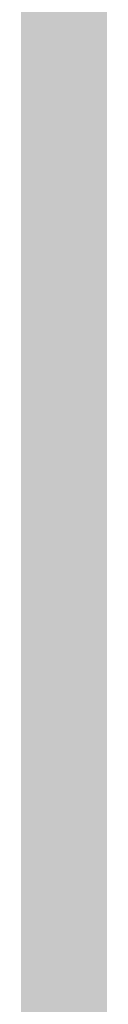
# Model space of a CAD drawing. Units: inches. Extents: x 2083 to 3317, y 1141 to 2115.
# Tile 173 of 256: x 3126.95825 to 3126.9594, y 1263.27402 to 1263.29018. Entities that reach past the tile are written whole.
import ezdxf

# ---------------------------------------------------------------- set-up
doc = ezdxf.new("R2010")
doc.units = ezdxf.units.IN
doc.layers.add('A-ANNO-DIMS', color=2, linetype='Continuous', lineweight=18)
doc.layers.add('A-WALL-PATT', color=251, linetype='Continuous', lineweight=13, true_color=0x636466)
doc.styles.get("Standard").update_dxf_attribs({"font": 'arial.ttf'})
doc.dimstyles.new('ISO-25', dxfattribs={"dimtxt": 12, "dimasz": 12, "dimexe": 1.25, "dimexo": 0.625, "dimtad": 1, "dimlunit": 3, "dimtxsty": 'Standard', "dimcen": 2.5, "dimadec": 0, "dimazin": 0, "dimtfac": 1, "dimtmove": 0, "dimatfit": 3, "dimfxl": 1, "dimarcsym": 0})

# ---------------------------------------------------------------- blocks, each defined once
blk = doc.blocks.new('*D26')
at = {"layer": 'A-ANNO-DIMS', "color": 0, "lineweight": -2, "transparency": 16777216}
for p, q in [((3088.985844, 1274.915092), (3088.985844, 1270.951963)), ((3111.240037, 1274.915092), (3111.240037, 1270.951963)), ((3076.985844, 1272.201963), (2840.262447, 1272.201963)), ((3111.240037, 1272.201963), (3088.985844, 1272.201963)), ((3123.240037, 1272.201963), (3135.240037, 1272.201963))]:
    blk.add_line(p, q, dxfattribs=at)
at = {"layer": 'A-ANNO-DIMS', "color": 0, "transparency": 16777216}
for points in [[(3076.985844, 1274.201963), (3076.985844, 1270.201963), (3088.985844, 1272.201963)], [(3123.240037, 1274.201963), (3123.240037, 1270.201963), (3111.240037, 1272.201963)]]:
    blk.add_solid(points, dxfattribs=at)
at = {"layer": 'Defpoints', "color": 0, "transparency": 16777216}
for p in [(3088.985844, 1275.540092), (3111.240037, 1275.540092), (3088.985844, 1272.201963)]:
    blk.add_point(p, dxfattribs=at)
at = {"layer": 'A-ANNO-DIMS', "color": 0, "transparency": 16777216, "insert": (2952.624146, 1279.031602), "char_height": 12, "attachment_point": 5}
blk.add_mtext('NIGHTSTAND 1\'-10 1/2" TYP.', dxfattribs=at)
blk = doc.blocks.new('*D27')
at = {"layer": 'A-ANNO-DIMS', "color": 0, "lineweight": -2, "transparency": 16777216}
for p, q in [((3114.578165, 1309.794285), (3114.578165, 1321.794285)), ((3111.865037, 1297.794285), (3115.828165, 1297.794285)), ((3114.578165, 1297.794285), (3114.578165, 1275.540092)), ((3111.865037, 1275.540092), (3115.828165, 1275.540092)), ((3114.578165, 1263.540092), (3114.578165, 1140.988591))]:
    blk.add_line(p, q, dxfattribs=at)
at = {"layer": 'A-ANNO-DIMS', "color": 0, "transparency": 16777216}
for points in [[(3112.578165, 1309.794285), (3116.578165, 1309.794285), (3114.578165, 1297.794285)], [(3112.578165, 1263.540092), (3116.578165, 1263.540092), (3114.578165, 1275.540092)]]:
    blk.add_solid(points, dxfattribs=at)
at = {"layer": 'Defpoints', "color": 0, "transparency": 16777216}
for p in [(3111.240037, 1297.794285), (3111.240037, 1275.540092), (3114.578165, 1275.540092)]:
    blk.add_point(p, dxfattribs=at)
at = {"layer": 'A-ANNO-DIMS', "color": 0, "transparency": 16777216, "insert": (3107.748527, 1196.264342), "char_height": 12, "attachment_point": 5, "rotation": 90}
blk.add_mtext('1\'-10 1/2" TYP.', dxfattribs=at)

msp = doc.modelspace()

# ---------------------------------------------------------------- hatches: boundary and pattern name
at = {"layer": 'A-WALL-PATT'}
h = msp.add_hatch(color=256, dxfattribs=at)
h.dxf.hatch_style = 1
h.paths.add_polyline_path([(3126.959783, 2020.76136), (2748.959783, 2020.76136), (2604.959783, 2020.76136), (2226.959783, 2020.76136), (2226.959783, 1702.76136), (2466.959783, 1702.76136), (2466.959783, 1582.76136), (2418.959783, 1582.76136), (2418.959783, 1477.76136), (2226.959783, 1477.76136), (2226.959783, 1263.26136), (2544.959783, 1263.26136), (2544.959783, 1411.76136), (2604.959783, 1411.76136), (2685.959783, 1411.76136), (2685.959783, 1420.76136), (2604.959783, 1420.76136), (2604.959783, 1573.76136), (2604.959783, 1702.76136), (2604.959783, 2011.76136), (2748.959783, 2011.76136), (2748.959783, 1702.76136), (2862.959783, 1702.76136), (2862.959783, 1621.76136), (2871.959783, 1621.76136), (2871.959783, 1702.76136), (2883.959783, 1702.76136), (2883.959783, 1706.939459, -0.026459), (2883.959783, 1711.76136), (2757.959783, 1711.76136), (2757.959783, 1807.76136), (2787.959783, 1807.76136), (2787.959783, 1812.26136), (2757.959783, 1812.26136), (2757.959783, 2011.76136), (2877.959783, 2011.76136), (2877.959783, 1812.26136), (2847.959783, 1812.26136), (2847.959783, 1807.76136), (2889.835742, 1807.76136), (2889.835742, 1812.26136), (2882.459783, 1812.26136), (2882.459783, 2011.76136), (3117.959783, 2011.76136), (3117.959783, 1812.26136), (2937.835742, 1812.26136), (2937.835742, 1807.76136), (2995.709783, 1807.76136), (2995.709783, 1796.117666), (3000.209783, 1796.117666), (3000.209783, 1807.76136), (3117.959783, 1807.76136), (3117.959783, 1711.76136), (3000.209783, 1711.76136), (3000.209783, 1760.117666), (2998.572705, 1760.117666, -0.020711), (2995.709783, 1760.117666), (2995.709783, 1711.76136), (2931.959783, 1711.76136), (2931.959783, 1702.76136), (3126.959783, 1702.76136)])
h.paths.add_polyline_path([(2471.459783, 2011.76136), (2471.459783, 1810.01136), (2462.716936, 1810.01136), (2462.716936, 1805.51136), (2505.959783, 1805.51136), (2505.959783, 1810.01136), (2475.959783, 1810.01136), (2475.959783, 2011.76136), (2595.959783, 2011.76136), (2595.959783, 1810.01136), (2565.959783, 1810.01136), (2565.959783, 1805.51136), (2595.959783, 1805.51136), (2595.959783, 1711.76136), (2235.959783, 1711.76136), (2235.959783, 1805.51136), (2353.709783, 1805.51136), (2353.709783, 1796.054162), (2358.209783, 1796.054162), (2358.209783, 1805.51136), (2414.716936, 1805.51136), (2414.716936, 1810.01136), (2235.959783, 1810.01136), (2235.959783, 2011.76136)], flags=16)
h.paths.add_polyline_path([(2270.204734, 1994.610008), (2270.204734, 1970.610008), (2246.204734, 1970.610008), (2246.204734, 1994.610008)], flags=0)
edge = h.paths.add_edge_path(flags=0)
edge.add_ellipse((2332.027391, 1899.798176), major_axis=(-3.042994, 3.042994), ratio=0.16825245, start_angle=-161.332166, end_angle=-156.307114, ccw=False)
edge.add_ellipse((2333.082037, 1898.74353), major_axis=(-1.054646, 1.054646), ratio=0.4535321, start_angle=-123.371019, end_angle=-94.159107)
edge = h.paths.add_edge_path(flags=0)
edge.add_ellipse((2332.027391, 1968.87629), major_axis=(3.042994, 3.042994), ratio=0.16825245, start_angle=18.667834, end_angle=23.692886)
edge.add_spline(control_points=[(2332.925596, 1970.691105), (2332.226768, 1970.3361), (2330.893709, 1969.658905), (2328.41308, 1970.932138), (2327.203934, 1967.748712), (2324.709596, 1969.955589), (2322.532822, 1967.012354), (2320.012846, 1971.295812), (2317.680308, 1968.157845), (2316.040526, 1967.102047), (2315.426904, 1966.809602)], knot_values=[0, 0, 0, 0, 2.267059, 4.324559, 6.685584, 8.878641, 11.121502, 14.300359, 17.755284, 19.732645, 19.732645, 19.732645, 19.732645], degree=3, periodic=0)
edge.add_ellipse((2332.027391, 1968.87629), major_axis=(3.042994, 3.042994), ratio=0.16825245, start_angle=18.667834, end_angle=23.692886, ccw=False)
edge.add_ellipse((2333.082037, 1969.930936), major_axis=(1.054646, 1.054646), ratio=0.4535321, start_angle=56.628981, end_angle=85.840893, ccw=False)
edge = h.paths.add_edge_path(flags=0)
edge.add_spline(control_points=[(2296.428287, 1967.987908), (2293.627804, 1965.336314), (2287.703624, 1959.727094), (2299.74386, 1949.995699), (2294.532591, 1935.668528), (2290.573228, 1920.603512), (2293.394124, 1909.973691), (2296.185407, 1904.966543)], knot_values=[0.099185, 0.099185, 0.099185, 0.099185, 0.345301, 0.619822, 0.982653, 1.386093, 1.810555, 1.810555, 1.810555, 1.810555], degree=3, periodic=0)
edge.add_spline(control_points=[(2296.185407, 1904.966543), (2297.383582, 1902.6193), (2298.000969, 1901.949312), (2298.55297, 1901.468155)], knot_values=[0.006246, 0.006246, 0.006246, 0.006246, 0.055476, 0.055476, 0.055476, 0.055476], degree=3, periodic=0)
edge.add_spline(control_points=[(2298.55297, 1901.468155), (2297.258612, 1900.923224), (2295.225294, 1900.232126), (2293.060229, 1900.614205), (2292.101423, 1900.788415), (2292.089578, 1900.790568)], knot_values=[0.312835, 0.312835, 0.312835, 0.312835, 0.40178, 0.474987, 0.475903, 0.475903, 0.475903, 0.475903], degree=3, periodic=0)
edge.add_arc((2292.793646, 1904.664109), 3.937008, 215.420897, 259.698179, ccw=False)
edge.add_spline(control_points=[(2289.585314, 1902.382304), (2289.476652, 1902.535087), (2289.36848, 1902.688035), (2289.260865, 1902.84117)], knot_values=[0.102872, 0.102872, 0.102872, 0.102872, 0.116896, 0.116896, 0.116896, 0.116896], degree=3, periodic=0)
edge.add_spline(control_points=[(2289.260865, 1902.84117), (2288.686604, 1902.550192), (2287.640048, 1902.019902), (2285.881337, 1901.873954), (2283.852972, 1901.504352), (2281.719987, 1899.710538), (2278.466991, 1899.492942), (2276.157136, 1901.883202), (2272.258953, 1899.804071), (2267.777605, 1901.843183), (2262.243882, 1900.184033), (2257.414927, 1901.782061), (2254.318374, 1900.72612), (2253.178285, 1900.337343)], knot_values=[0, 0, 0, 0, 1.907977, 3.477176, 5.261074, 7.972851, 11.680248, 13.717921, 16.939592, 22.789562, 27.502503, 33.595215, 37.145618, 37.145618, 37.145618, 37.145618], degree=3, periodic=0)
edge.add_line((2253.178285, 1900.337343), (2250.24424, 1902.84117))
edge.add_line((2250.24424, 1902.84117), (2250.24424, 1965.833296))
edge.add_line((2250.24424, 1965.833296), (2253.178285, 1968.337123))
edge.add_spline(control_points=[(2253.178285, 1968.337123), (2254.318374, 1967.948346), (2257.414927, 1966.892405), (2262.243882, 1968.490433), (2267.777605, 1966.831283), (2271.52673, 1968.537217), (2273.875914, 1967.828289), (2274.206701, 1967.727642)], knot_values=[0, 0, 0, 0, 0.09018, 0.244935, 0.364644, 0.513233, 0.537855, 0.537855, 0.537855, 0.537855], degree=3, periodic=0)
edge.add_arc((2274.352887, 1963.793349), 3.937008, 72.051134, 92.127949, ccw=False)
edge.add_arc((2281.296933, 1985.230003), 18.596298, 252.0511336, 288.5657217)
edge.add_arc((2292.316717, 1956.02888), 12.646081, 71.0267879, 113.7782184, ccw=False)
edge = h.paths.add_edge_path(flags=0)
edge.add_spline(control_points=[(2274.899415, 1951.856195), (2275.066156, 1951.616592), (2275.232687, 1951.376588), (2275.397987, 1951.135855)], knot_values=[1.409916, 1.409916, 1.409916, 1.409916, 1.43159, 1.43159, 1.43159, 1.43159], degree=3, periodic=0)
edge.add_spline(control_points=[(2275.397987, 1951.135855), (2275.792106, 1950.561885), (2276.179231, 1949.983774), (2276.545546, 1949.397103)], knot_values=[1.358238, 1.358238, 1.358238, 1.358238, 1.409916, 1.409916, 1.409916, 1.409916], degree=3, periodic=0)
edge.add_line((2276.545546, 1949.397103), (2277.437289, 1947.862185))
edge.add_spline(control_points=[(2277.437289, 1947.862185), (2276.303834, 1945.673115), (2274.639698, 1942.426882), (2274.631615, 1938.0939), (2272.799124, 1930.85155), (2274.356426, 1943.897046), (2275.947681, 1947.923356), (2276.545546, 1949.397103)], knot_values=[0.005632, 0.005632, 0.005632, 0.005632, 0.186014, 0.266002, 0.357087, 0.59639, 0.739732, 0.739732, 0.739732, 0.739732], degree=3, periodic=0)
edge.add_spline(control_points=[(2276.545546, 1949.397103), (2276.179231, 1949.983774), (2275.792106, 1950.561885), (2275.397987, 1951.135855)], knot_values=[1.358238, 1.358238, 1.358238, 1.358238, 1.409916, 1.409916, 1.409916, 1.409916], degree=3, periodic=0)
edge.add_spline(control_points=[(2275.397987, 1951.135855), (2274.9425, 1950.080452), (2274.20776, 1948.025272), (2273.934602, 1944.851477), (2272.468534, 1937.627489), (2273.466216, 1945.696466), (2274.700615, 1951.059472), (2274.899415, 1951.856195)], knot_values=[0.104364, 0.104364, 0.104364, 0.104364, 0.189636, 0.269624, 0.36071, 0.600013, 0.644622, 0.644622, 0.644622, 0.644622], degree=3, periodic=0)
h.paths.add_polyline_path([(2269.167514, 1963.127573, -0.357527), (2268.170633, 1960.97637, -0.092561), (2268.170633, 1939.436325, -0.357527), (2269.167514, 1937.285122, -0.357527), (2267.01631, 1938.282002, -0.164785), (2254.685581, 1938.282002, -0.357527), (2252.534378, 1937.285122, -0.357527), (2253.531259, 1939.436325, -0.092561), (2253.531259, 1960.97637, -0.357527), (2252.534378, 1963.127573, -0.357527), (2254.685581, 1962.130692, -0.164785), (2267.01631, 1962.130692, -0.357527)], flags=0)
h.paths.add_polyline_path([(2248.874068, 1967.8018), (2248.874068, 1957.02771), (2249.457783, 1957.02771), (2249.457783, 1911.646756), (2248.874068, 1911.646756), (2248.874068, 1900.872666), (2246.511863, 1900.872666, 0.197327), (2244.149658, 1902.456873), (2244.149658, 1966.217592, 0.197327), (2246.511863, 1967.8018)], flags=0)
h.paths.add_polyline_path([(2269.167514, 1931.389344, -0.357527), (2268.170633, 1929.238141, -0.092561), (2268.170633, 1907.698096, -0.357527), (2269.167514, 1905.546893, -0.357527), (2267.01631, 1906.543774, -0.164785), (2254.685581, 1906.543774, -0.357527), (2252.534378, 1905.546893, -0.357527), (2253.531259, 1907.698096, -0.092561), (2253.531259, 1929.238141, -0.357527), (2252.534378, 1931.389344, -0.357527), (2254.685581, 1930.392463, -0.164785), (2267.01631, 1930.392463, -0.357527)], flags=0)
edge = h.paths.add_edge_path(flags=0)
edge.add_spline(control_points=[(2276.196858, 1906.723702), (2276.168144, 1909.028928), (2276.114049, 1913.371852), (2270.598417, 1924.924978), (2273.905175, 1919.012779), (2275.921711, 1916.262063), (2275.47457, 1912.402149), (2277.257874, 1910.380621), (2276.696044, 1908.225036), (2276.646218, 1906.813023), (2276.617825, 1906.008407)], knot_values=[0, 0, 0, 0, 8.61026, 16.221274, 18.843057, 23.804898, 27.440828, 29.356102, 31.203478, 33.650687, 33.650687, 33.650687, 33.650687], degree=3, periodic=0)
edge.add_spline(control_points=[(2276.617825, 1906.008407), (2276.623313, 1905.624144), (2276.497738, 1904.628661), (2275.441779, 1903.854725), (2274.937314, 1903.08045), (2274.85908, 1902.84117)], knot_values=[0.156488, 0.156488, 0.156488, 0.156488, 0.184398, 0.231376, 0.250598, 0.250598, 0.250598, 0.250598], degree=3, periodic=0)
edge.add_line((2274.85908, 1902.84117), (2276.50598, 1902.84117))
edge.add_spline(control_points=[(2276.50598, 1902.84117), (2276.788308, 1903.08494), (2277.665071, 1904.125196), (2278.249538, 1904.340738), (2277.653872, 1908.527387), (2278.15567, 1906.227808), (2278.100464, 1905.285948), (2278.846675, 1904.069005), (2277.856785, 1903.414948), (2277.874191, 1902.99105), (2277.903562, 1902.84117)], knot_values=[0.059574, 0.059574, 0.059574, 0.059574, 0.080753, 0.103741, 0.16972, 0.176036, 0.207137, 0.240474, 0.262341, 0.27366, 0.27366, 0.27366, 0.27366], degree=3, periodic=0)
edge.add_line((2277.903562, 1902.84117), (2280.029825, 1902.84117))
edge.add_spline(control_points=[(2280.029825, 1902.84117), (2279.888221, 1903.088398), (2279.499257, 1903.981551), (2280.152284, 1905.939349), (2278.103615, 1909.657757), (2279.762395, 1907.185285), (2280.3279, 1904.874861), (2280.485109, 1903.48959), (2281.463269, 1903.249432), (2281.758343, 1902.936497), (2281.834036, 1902.84117)], knot_values=[0.013856, 0.013856, 0.013856, 0.013856, 0.034874, 0.088867, 0.107879, 0.126738, 0.158714, 0.193757, 0.217487, 0.226722, 0.226722, 0.226722, 0.226722], degree=3, periodic=0)
edge.add_spline(control_points=[(2281.834036, 1902.84117), (2281.787535, 1902.826703), (2281.647022, 1902.782988), (2281.395527, 1902.85949), (2281.088077, 1902.985242), (2280.720683, 1903.060902), (2280.333451, 1903.025726), (2280.124767, 1902.898879), (2280.029825, 1902.84117)], knot_values=[0, 0, 0, 0, 0.14413, 0.435517, 0.749276, 1.153046, 1.548371, 1.878348, 1.878348, 1.878348, 1.878348], degree=3, periodic=0)
edge.add_line((2280.029825, 1902.84117), (2277.903562, 1902.84117))
edge.add_spline(control_points=[(2277.903562, 1902.84117), (2277.892855, 1902.795855), (2277.865396, 1902.679637), (2277.607479, 1902.687483), (2277.27405, 1902.8007), (2276.837921, 1902.619775), (2276.583807, 1902.789261), (2276.50598, 1902.84117)], knot_values=[0, 0, 0, 0, 0.127189, 0.326199, 0.628009, 1.24357, 1.515331, 1.515331, 1.515331, 1.515331], degree=3, periodic=0)
edge.add_line((2276.50598, 1902.84117), (2274.85908, 1902.84117))
edge.add_spline(control_points=[(2274.85908, 1902.84117), (2274.814437, 1902.898587), (2274.72513, 1903.013446), (2274.493477, 1903.118968), (2274.244285, 1902.960539), (2273.937121, 1903.184942), (2273.614039, 1902.983143), (2273.408316, 1902.883045), (2273.322254, 1902.84117)], knot_values=[0, 0, 0, 0, 0.21843, 0.436957, 0.687977, 0.990379, 1.398396, 1.69185, 1.69185, 1.69185, 1.69185], degree=3, periodic=0)
edge.add_spline(control_points=[(2273.322254, 1902.84117), (2273.61674, 1903.445692), (2274.273998, 1904.538253), (2276.027239, 1904.573702), (2276.206963, 1906.583637), (2276.196858, 1906.723702)], knot_values=[0.012227, 0.012227, 0.012227, 0.012227, 0.059472, 0.106218, 0.134458, 0.134458, 0.134458, 0.134458], degree=3, periodic=0)
h.paths.add_polyline_path([(2270.776054, 1897.789828), (2270.776054, 1873.789828), (2246.776054, 1873.789828), (2246.776054, 1897.789828)], flags=0)
h.paths.add_polyline_path([(2353.709783, 1760.005059), (2353.709783, 1760.054162), (2358.209783, 1760.054162, -0.033729)], flags=0)
h.paths.add_polyline_path([(2321.819119, 1737.529186), (2341.995327, 1737.529186, -0.414214), (2343.203273, 1736.321241), (2343.203273, 1721.020596, -0.414214), (2341.995327, 1719.812651), (2321.819119, 1719.812651, -0.414214), (2320.611173, 1721.020596), (2320.611173, 1736.321241, -0.414214)], flags=0)
h.paths.add_polyline_path([(2324.23501, 1736.321241), (2339.579436, 1736.321241, -0.414214), (2341.995327, 1733.905349), (2341.995327, 1725.44973, -0.414214), (2339.579436, 1723.033839), (2333.680588, 1723.033839), (2333.845317, 1722.045467, -0.870646), (2335.425399, 1721.825893, -0.767327), (2333.922694, 1721.423245), (2331.291024, 1721.423245, -0.767327), (2329.788319, 1721.825893, -0.870646), (2331.368401, 1722.045467), (2331.53313, 1723.033839), (2324.23501, 1723.033839, -0.414214), (2321.819119, 1725.44973), (2321.819119, 1733.905349, -0.414214)], flags=0)
h.paths.add_polyline_path([(2570.483789, 1928.615444), (2589.683789, 1928.615444), (2590.168829, 1928.615444), (2590.168829, 1904.993397), (2570.483789, 1904.993397)], flags=0)
h.paths.add_polyline_path([(2574.447324, 1927.263822, -1), (2572.828836, 1927.263822, -1)], flags=0)
h.paths.add_polyline_path([(2573.089867, 1926.940877), (2573.925032, 1927.776042), (2574.147743, 1927.553332), (2573.312577, 1926.718166)], flags=0)
h.paths.add_polyline_path([(2578.779065, 1919.729618, -1), (2571.591663, 1919.729618, -1)], flags=0)
h.paths.add_polyline_path([(2578.385364, 1919.729618, -1), (2571.985364, 1919.729618, -1)], flags=0)
h.paths.add_polyline_path([(2331.595764, 1729.476216, -1), (2333.617954, 1729.476216, -1)], flags=0)
h.paths.add_polyline_path([(2578.034228, 1927.263822, -1), (2576.41574, 1927.263822, -1)], flags=0)
h.paths.add_polyline_path([(2576.688851, 1927.531089), (2576.911562, 1927.753799), (2577.746728, 1926.918634), (2577.524017, 1926.695923)], flags=0)
h.paths.add_polyline_path([(2578.139065, 1909.859539, -1), (2572.231663, 1909.859539, -1)], flags=0)
h.paths.add_polyline_path([(2577.745364, 1909.859539, -1), (2572.625364, 1909.859539, -1)], flags=0)
h.paths.add_polyline_path([(2583.797718, 1927.263822, -1), (2582.179229, 1927.263822, -1)], flags=0)
h.paths.add_polyline_path([(2582.718649, 1927.753799), (2583.553814, 1926.918634), (2583.331103, 1926.695923), (2582.495938, 1927.531089)], flags=0)
h.paths.add_polyline_path([(2582.495938, 1927.531089), (2582.718649, 1927.753799), (2583.553814, 1926.918634), (2583.331103, 1926.695923)], flags=0)
h.paths.add_polyline_path([(2587.739065, 1920.529618, -1), (2581.831663, 1920.529618, -1)], flags=0)
h.paths.add_polyline_path([(2587.345364, 1920.529618, -1), (2582.225364, 1920.529618, -1)], flags=0)
h.paths.add_polyline_path([(2587.384622, 1927.263822, -1), (2585.766133, 1927.263822, -1)], flags=0)
h.paths.add_polyline_path([(2586.081993, 1926.980247), (2586.917158, 1927.815412), (2587.139869, 1927.592702), (2586.304703, 1926.757536)], flags=0)
h.paths.add_polyline_path([(2588.379065, 1910.659539, -1), (2581.191663, 1910.659539, -1)], flags=0)
h.paths.add_polyline_path([(2587.985364, 1910.659539, -1), (2581.585364, 1910.659539, -1)], flags=0)
h.paths.add_polyline_path([(2417.167729, 1729.477895), (2437.343937, 1729.477895, -0.414214), (2438.551883, 1728.26995), (2438.551883, 1712.969306, -0.414214), (2437.343937, 1711.76136), (2417.167729, 1711.76136, -0.414214), (2415.959783, 1712.969306), (2415.959783, 1728.26995, -0.414214)], flags=0)
h.paths.add_polyline_path([(2419.58362, 1728.26995), (2434.928046, 1728.26995, -0.414214), (2437.343937, 1725.854059), (2437.343937, 1717.39844, -0.414214), (2434.928046, 1714.982548), (2429.029199, 1714.982548), (2429.193927, 1713.994176, -0.870646), (2430.774009, 1713.774603, -0.767327), (2429.271304, 1713.371954), (2426.639634, 1713.371954, -0.767327), (2425.136929, 1713.774603, -0.870646), (2426.717011, 1713.994176), (2426.88174, 1714.982548), (2419.58362, 1714.982548, -0.414214), (2417.167729, 1717.39844), (2417.167729, 1725.854059, -0.414214)], flags=0)
h.paths.add_polyline_path([(2419.58362, 1728.26995), (2434.928046, 1728.26995, -0.414214), (2437.343937, 1725.854059), (2437.343937, 1717.39844, -0.414214), (2434.928046, 1714.982548), (2429.029199, 1714.982548), (2428.358118, 1719.009034), (2427.552821, 1719.009034), (2426.88174, 1714.982548), (2419.58362, 1714.982548, -0.414214), (2417.167729, 1717.39844), (2417.167729, 1725.854059, -0.414214)], flags=0)
h.paths.add_polyline_path([(2426.944374, 1721.424925, -1), (2428.966564, 1721.424925, -1)], flags=0)
h.paths.add_polyline_path([(2475.959783, 1702.76136), (2595.959783, 1702.76136), (2595.959783, 1582.76136), (2475.959783, 1582.76136)], flags=16)
h.paths.add_polyline_path([(2427.959783, 1573.76136), (2595.959783, 1573.76136), (2595.959783, 1468.76136), (2595.959783, 1420.76136), (2384.459783, 1420.76136), (2384.459783, 1468.76136), (2427.959783, 1468.76136)], flags=16)
h.paths.add_polyline_path([(2379.959783, 1468.76136), (2379.959783, 1420.76136), (2235.959783, 1420.76136), (2235.959783, 1468.76136)], flags=16)
h.paths.add_polyline_path([(2317.815996, 1466.695767), (2337.992205, 1466.695767, -0.414214), (2339.20015, 1465.487821), (2339.20015, 1450.187177, -0.414214), (2337.992205, 1448.979232), (2317.815996, 1448.979232, -0.414214), (2316.608051, 1450.187177), (2316.608051, 1465.487821, -0.414214)], flags=0)
h.paths.add_polyline_path([(2320.231887, 1465.487821), (2335.576313, 1465.487821, -0.414214), (2337.992205, 1463.07193), (2337.992205, 1454.616311, -0.414214), (2335.576313, 1452.20042), (2329.677466, 1452.20042), (2329.842195, 1451.212047, -0.870646), (2331.422276, 1450.992474, -0.767327), (2329.919571, 1450.589826), (2327.287902, 1450.589826, -0.767327), (2325.785197, 1450.992474, -0.870646), (2327.365278, 1451.212047), (2327.530007, 1452.20042), (2320.231887, 1452.20042, -0.414214), (2317.815996, 1454.616311), (2317.815996, 1463.07193, -0.414214)], flags=0)
h.paths.add_polyline_path([(2320.231887, 1465.487821), (2335.576313, 1465.487821, -0.414214), (2337.992205, 1463.07193), (2337.992205, 1454.616311, -0.414214), (2335.576313, 1452.20042), (2329.677466, 1452.20042), (2329.006385, 1456.226905), (2328.201088, 1456.226905), (2327.530007, 1452.20042), (2320.231887, 1452.20042, -0.414214), (2317.815996, 1454.616311), (2317.815996, 1463.07193, -0.414214)], flags=0)
h.paths.add_polyline_path([(2327.592641, 1458.642796, -1), (2329.614832, 1458.642796, -1)], flags=0)
h.paths.add_polyline_path([(2244.411744, 1433.340453), (2241.920945, 1433.340453, -0.414214), (2240.017856, 1435.243542), (2240.017856, 1440.952808, -0.414211), (2241.920925, 1442.855897), (2244.411744, 1442.855897, -1.976472)], flags=0)
h.paths.add_polyline_path([(2245.356888, 1434.397536, -0.414214), (2245.356888, 1441.798814, -2.144098)], flags=0)
h.paths.add_polyline_path([(2535.959783, 1416.26136), (2535.959783, 1272.26136), (2235.959783, 1272.26136), (2235.959783, 1416.26136)], flags=16)
h.paths.add_polyline_path([(2260.119561, 1384.292841), (2260.119561, 1362.038649), (2237.865369, 1362.038649), (2237.865369, 1384.292841)], flags=0)
edge = h.paths.add_edge_path(flags=0)
edge.add_line((2318.251847, 1362.093298), (2318.145797, 1362.000973))
edge.add_ellipse((2317.445116, 1360.431044), major_axis=(2.82164, 2.82164), ratio=0.16825245, start_angle=18.667834, end_angle=20.948127, ccw=False)
edge.add_ellipse((2318.423045, 1361.408974), major_axis=(0.977929, 0.977929), ratio=0.4535321, start_angle=56.628981, end_angle=70.226201, ccw=False)
edge = h.paths.add_edge_path(flags=0)
edge.add_line((2319.10737, 1295.571078), (2319.015044, 1295.677128))
edge.add_ellipse((2317.445116, 1296.377809), major_axis=(-2.82164, 2.82164), ratio=0.16825245, start_angle=-161.332166, end_angle=-159.051873, ccw=False)
edge.add_ellipse((2318.423045, 1295.39988), major_axis=(-0.977929, 0.977929), ratio=0.4535321, start_angle=-123.371019, end_angle=-109.773799)
edge = h.paths.add_edge_path(flags=0)
edge.add_spline(control_points=[(2284.210349, 1301.170219), (2284.580688, 1300.444719), (2284.891189, 1299.892024), (2285.159553, 1299.461018)], knot_values=[0.039066, 0.039066, 0.039066, 0.039066, 0.055476, 0.055476, 0.055476, 0.055476], degree=3, periodic=0)
edge.add_line((2285.159553, 1299.461018), (2284.210349, 1301.170219))
edge = h.paths.add_edge_path(flags=0)
edge.add_line((2280.412458, 1297.298013), (2283.369991, 1297.036122))
edge.add_line((2283.369991, 1297.036122), (2286.40569, 1297.92631))
edge.add_spline(control_points=[(2286.40569, 1297.92631), (2285.305487, 1297.463119), (2284.344777, 1297.129151), (2283.369991, 1297.036122)], knot_values=[0.394369, 0.394369, 0.394369, 0.394369, 0.475903, 0.475903, 0.475903, 0.475903], degree=3, periodic=0)
edge.add_spline(control_points=[(2283.369991, 1297.036122), (2283.28139, 1297.027666), (2282.316289, 1296.957336), (2281.312502, 1297.134479), (2280.423441, 1297.296016), (2280.412458, 1297.298013)], knot_values=[0.312835, 0.312835, 0.312835, 0.312835, 0.320246, 0.393453, 0.394369, 0.394369, 0.394369, 0.394369], degree=3, periodic=0)
edge = h.paths.add_edge_path(flags=0)
edge.add_line((2284.435561, 1359.607285), (2280.446291, 1355.328047))
edge.add_line((2280.446291, 1355.328047), (2279.579987, 1351.017754))
edge.add_line((2279.579987, 1351.017754), (2282.412974, 1346.580433))
edge.add_spline(control_points=[(2282.412974, 1346.580433), (2283.153331, 1345.589236), (2284.252896, 1344.028897), (2284.801037, 1342.387167), (2284.935162, 1341.805544)], knot_values=[1.240098, 1.240098, 1.240098, 1.240098, 1.332892, 1.382712, 1.382712, 1.382712, 1.382712], degree=3, periodic=0)
edge.add_spline(control_points=[(2284.935162, 1341.805544), (2285.319108, 1340.1406), (2285.233029, 1338.409204), (2284.909938, 1336.654122)], knot_values=[1.097484, 1.097484, 1.097484, 1.097484, 1.240098, 1.240098, 1.240098, 1.240098], degree=3, periodic=0)
edge.add_spline(control_points=[(2284.909938, 1336.654122), (2284.586848, 1334.89904), (2284.026745, 1333.120272), (2283.462644, 1331.360585)], knot_values=[0.95487, 0.95487, 0.95487, 0.95487, 1.097484, 1.097484, 1.097484, 1.097484], degree=3, periodic=0)
edge.add_line((2283.462644, 1331.360585), (2281.890376, 1326.153357))
edge.add_line((2281.890376, 1326.153357), (2280.756259, 1321.056089))
edge.add_line((2280.756259, 1321.056089), (2280.299205, 1316.001977))
edge.add_line((2280.299205, 1316.001977), (2280.715933, 1310.950068))
edge.add_line((2280.715933, 1310.950068), (2282.028094, 1305.972137))
edge.add_line((2282.028094, 1305.972137), (2284.210349, 1301.170219))
edge.add_spline(control_points=[(2284.210349, 1301.170219), (2283.340731, 1302.730185), (2282.611904, 1304.336493), (2282.028094, 1305.972137)], knot_values=[0.099185, 0.099185, 0.099185, 0.099185, 0.241799, 0.241799, 0.241799, 0.241799], degree=3, periodic=0)
edge.add_spline(control_points=[(2282.028094, 1305.972137), (2281.444283, 1307.60778), (2281.005489, 1309.272759), (2280.715933, 1310.950068)], knot_values=[0.241799, 0.241799, 0.241799, 0.241799, 0.384413, 0.384413, 0.384413, 0.384413], degree=3, periodic=0)
edge.add_spline(control_points=[(2280.715933, 1310.950068), (2280.433241, 1312.587613), (2280.289386, 1314.276959), (2280.298894, 1315.962032), (2280.299205, 1316.001977)], knot_values=[0.384413, 0.384413, 0.384413, 0.384413, 0.523647, 0.527028, 0.527028, 0.527028, 0.527028], degree=3, periodic=0)
edge.add_spline(control_points=[(2280.299205, 1316.001977), (2280.312326, 1317.686955), (2280.477871, 1319.367926), (2280.756259, 1321.056089)], knot_values=[0.527028, 0.527028, 0.527028, 0.527028, 0.669642, 0.669642, 0.669642, 0.669642], degree=3, periodic=0)
edge.add_spline(control_points=[(2280.756259, 1321.056089), (2281.034648, 1322.744252), (2281.42588, 1324.439608), (2281.890376, 1326.153357)], knot_values=[0.669642, 0.669642, 0.669642, 0.669642, 0.812256, 0.812256, 0.812256, 0.812256], degree=3, periodic=0)
edge.add_spline(control_points=[(2281.890376, 1326.153357), (2282.264383, 1327.533251), (2282.78787, 1329.26181), (2283.352751, 1331.01778), (2283.462644, 1331.360585)], knot_values=[0.812256, 0.812256, 0.812256, 0.812256, 0.927087, 0.95487, 0.95487, 0.95487, 0.95487], degree=3, periodic=0)
edge.add_line((2283.462644, 1331.360585), (2284.909938, 1336.654122))
edge.add_line((2284.909938, 1336.654122), (2284.935162, 1341.805544))
edge.add_line((2284.935162, 1341.805544), (2282.412974, 1346.580433))
edge.add_spline(control_points=[(2282.412974, 1346.580433), (2281.275127, 1348.103792), (2280.078447, 1349.570318), (2279.579987, 1351.017754)], knot_values=[1.382712, 1.382712, 1.382712, 1.382712, 1.525326, 1.525326, 1.525326, 1.525326], degree=3, periodic=0)
edge.add_spline(control_points=[(2279.579987, 1351.017754), (2279.443282, 1351.414721), (2279.136312, 1352.856922), (2279.73519, 1354.290385), (2280.446291, 1355.328047)], knot_values=[1.525326, 1.525326, 1.525326, 1.525326, 1.564439, 1.667941, 1.667941, 1.667941, 1.667941], degree=3, periodic=0)
edge.add_spline(control_points=[(2280.446291, 1355.328047), (2281.426113, 1356.757835), (2282.930837, 1358.18256), (2284.435561, 1359.607285)], knot_values=[1.667941, 1.667941, 1.667941, 1.667941, 1.810555, 1.810555, 1.810555, 1.810555], degree=3, periodic=0)
edge.add_arc((2280.623075, 1348.518181), 11.72618, 71.0267879, 113.7782184)
edge.add_arc((2270.404892, 1375.595156), 17.243567, 252.0511336, 288.5657217, ccw=False)
edge.add_arc((2263.965969, 1355.717847), 3.650622, 72.051134, 92.127949)
edge.add_arc((2263.965969, 1355.717847), 3.650622, 92.127949, 177.98513)
edge.add_spline(control_points=[(2260.317604, 1355.846199), (2260.260417, 1354.220668), (2260.551278, 1350.186547), (2262.999344, 1346.766251), (2264.472741, 1344.649024)], knot_values=[1.43159, 1.43159, 1.43159, 1.43159, 1.564144, 1.770695, 1.770695, 1.770695, 1.770695], degree=3, periodic=0)
edge.add_line((2264.472741, 1344.649024), (2264.93559, 1343.98253))
edge.add_spline(control_points=[(2263.801044, 1340.248105), (2263.843238, 1340.514088), (2264.067244, 1341.756465), (2264.512693, 1343.002453), (2264.935047, 1343.981083)], knot_values=[0.53657, 0.53657, 0.53657, 0.53657, 0.559349, 0.644622, 0.644622, 0.644622, 0.644622], degree=3, periodic=0)
edge.add_spline(control_points=[(2264.935047, 1343.981083), (2265.117771, 1343.714975), (2265.298875, 1343.447906), (2265.476756, 1343.179365)], knot_values=[1.384077, 1.384077, 1.384077, 1.384077, 1.409916, 1.409916, 1.409916, 1.409916], degree=3, periodic=0)
edge.add_spline(control_points=[(2265.476756, 1343.179365), (2265.654637, 1342.910823), (2265.829296, 1342.64081), (2265.99913, 1342.368812)], knot_values=[1.358238, 1.358238, 1.358238, 1.358238, 1.384077, 1.384077, 1.384077, 1.384077], degree=3, periodic=0)
edge.add_line((2265.99913, 1342.368812), (2266.826006, 1340.945547))
edge.add_spline(control_points=[(2266.826006, 1340.945547), (2268.894401, 1337.089691), (2271.398173, 1325.843001), (2270.516164, 1310.568557), (2275.919376, 1301.860609), (2277.789511, 1299.19945)], knot_values=[0.116896, 0.116896, 0.116896, 0.116896, 0.472987, 1.050969, 1.313793, 1.313793, 1.313793, 1.313793], degree=3, periodic=0)
edge.add_spline(control_points=[(2277.789511, 1299.19945), (2277.839405, 1299.128452), (2277.889428, 1299.057498), (2277.939572, 1298.986584)], knot_values=[0.109884, 0.109884, 0.109884, 0.109884, 0.116896, 0.116896, 0.116896, 0.116896], degree=3, periodic=0)
edge.add_line((2277.939572, 1298.986584), (2277.788849, 1299.199114))
edge.add_spline(control_points=[(2277.788849, 1299.199114), (2277.256582, 1298.929414), (2276.28635, 1298.437902), (2275.039352, 1298.334419), (2274.38333, 1298.238895), (2274.215254, 1298.209338)], knot_values=[33.12187, 33.12187, 33.12187, 33.12187, 35.029056, 36.598255, 37.144827, 37.144827, 37.144827, 37.144827], degree=3, periodic=0)
edge.add_line((2274.215254, 1298.209338), (2273.073147, 1297.892961))
edge.add_spline(control_points=[(2273.073147, 1297.892961), (2272.322936, 1297.579784), (2271.039151, 1296.510508), (2269.248395, 1296.226062), (2268.4231, 1296.374654)], knot_values=[26.532584, 26.532584, 26.532584, 26.532584, 29.198919, 31.839101, 31.839101, 31.839101, 31.839101], degree=3, periodic=0)
edge.add_line((2268.4231, 1296.374654), (2263.878501, 1297.457534))
edge.add_spline(control_points=[(2263.878501, 1297.457534), (2263.556077, 1297.359435), (2261.860306, 1296.838694), (2260.23878, 1297.282407), (2258.933454, 1297.516461)], knot_values=[15.919551, 15.919551, 15.919551, 15.919551, 16.939592, 21.226067, 21.226067, 21.226067, 21.226067], degree=3, periodic=0)
edge.add_line((2258.933454, 1297.516461), (2254.055233, 1297.32901))
edge.add_spline(control_points=[(2254.055233, 1297.32901), (2253.755525, 1297.295815), (2252.113683, 1297.165174), (2250.461869, 1297.544221), (2249.129686, 1297.667882)], knot_values=[5.306517, 5.306517, 5.306517, 5.306517, 6.276435, 10.613034, 10.613034, 10.613034, 10.613034], degree=3, periodic=0)
edge.add_line((2249.129686, 1297.667882), (2244.33165, 1296.877756))
edge.add_line((2244.33165, 1296.877756), (2241.611033, 1299.19945))
edge.add_line((2241.611033, 1299.19945), (2241.611033, 1357.609404))
edge.add_line((2241.611033, 1357.609404), (2244.33165, 1359.931097))
edge.add_line((2244.33165, 1359.931097), (2252.728823, 1359.542692))
edge.add_spline(control_points=[(2252.728823, 1359.542692), (2252.870939, 1359.54644), (2253.30574, 1359.548172), (2253.739845, 1359.514274), (2254.031742, 1359.482426)], knot_values=[0.233291, 0.233291, 0.233291, 0.233291, 0.244935, 0.268927, 0.268927, 0.268927, 0.268927], degree=3, periodic=0)
edge.add_line((2254.031742, 1359.482426), (2259.58719, 1359.41639))
edge.add_spline(control_points=[(2259.58719, 1359.41639), (2260.677068, 1359.628503), (2262.073197, 1359.897003), (2263.523692, 1359.459278), (2263.830417, 1359.365952)], knot_values=[0.422516, 0.422516, 0.422516, 0.422516, 0.513233, 0.537855, 0.537855, 0.537855, 0.537855], degree=3, periodic=0)
edge.add_arc((2263.965969, 1355.717847), 3.650622, 72.051134, 92.127949, ccw=False)
edge.add_arc((2270.404892, 1375.595156), 17.243567, 252.0511336, 288.5657217)
edge.add_arc((2280.623075, 1348.518181), 11.72618, 71.0267879, 113.7782184, ccw=False)
h.paths.add_polyline_path([(2240.34053, 1359.434715), (2240.34053, 1349.444353), (2240.881785, 1349.444353), (2240.881785, 1307.3645), (2240.34053, 1307.3645), (2240.34053, 1297.374138), (2238.150157, 1297.374138, 0.197327), (2235.959783, 1298.843108), (2235.959783, 1357.965746, 0.197327), (2238.150157, 1359.434715)], flags=0)
h.paths.add_polyline_path([(2259.15779, 1355.1005, -0.357527), (2258.233425, 1353.10578, -0.092561), (2258.233425, 1333.132601, -0.357527), (2259.15779, 1331.13788, -0.357527), (2257.16307, 1332.062246, -0.164785), (2245.729302, 1332.062246, -0.357527), (2243.734582, 1331.13788, -0.357527), (2244.658947, 1333.132601, -0.092561), (2244.658947, 1353.10578, -0.357527), (2243.734582, 1355.1005, -0.357527), (2245.729302, 1354.176135, -0.164785), (2257.16307, 1354.176135, -0.357527)], flags=0)
edge = h.paths.add_edge_path(flags=0)
edge.add_line((2265.99913, 1342.368812), (2266.826006, 1340.945547))
edge.add_line((2266.826006, 1340.945547), (2265.307557, 1337.814066))
edge.add_line((2265.307557, 1337.814066), (2264.358232, 1334.652939))
edge.add_line((2264.358232, 1334.652939), (2264.262012, 1333.799705))
edge.add_spline(control_points=[(2264.262012, 1333.799705), (2264.208357, 1333.187055), (2264.16206, 1332.365525), (2264.007144, 1331.413933), (2263.969049, 1331.201834)], knot_values=[0.464444, 0.464444, 0.464444, 0.464444, 0.516691, 0.531608, 0.531608, 0.531608, 0.531608], degree=3, periodic=0)
edge.add_spline(control_points=[(2263.969049, 1331.201834), (2263.774535, 1330.118873), (2263.42437, 1328.790839), (2263.25742, 1328.530652), (2263.234028, 1328.514612)], knot_values=[0.372682, 0.372682, 0.372682, 0.372682, 0.44885, 0.464444, 0.464444, 0.464444, 0.464444], degree=3, periodic=0)
edge.add_spline(control_points=[(2263.234028, 1328.514612), (2263.096382, 1328.420227), (2263.13117, 1329.301477), (2263.274953, 1330.615749)], knot_values=[0.280919, 0.280919, 0.280919, 0.280919, 0.372682, 0.372682, 0.372682, 0.372682], degree=3, periodic=0)
edge.add_spline(control_points=[(2263.274953, 1330.615749), (2263.418736, 1331.930022), (2263.671515, 1333.677318), (2263.969852, 1335.315027)], knot_values=[0.189157, 0.189157, 0.189157, 0.189157, 0.280919, 0.280919, 0.280919, 0.280919], degree=3, periodic=0)
edge.add_spline(control_points=[(2263.969852, 1335.315027), (2264.100496, 1336.032192), (2264.418783, 1337.621911), (2264.754848, 1338.86443), (2264.947419, 1339.491124)], knot_values=[0.097394, 0.097394, 0.097394, 0.097394, 0.137578, 0.189157, 0.189157, 0.189157, 0.189157], degree=3, periodic=0)
edge.add_spline(control_points=[(2264.947419, 1339.491124), (2265.290017, 1340.606055), (2265.644238, 1341.493996), (2265.99913, 1342.368812)], knot_values=[0.005632, 0.005632, 0.005632, 0.005632, 0.097394, 0.097394, 0.097394, 0.097394], degree=3, periodic=0)
h.paths.add_polyline_path([(2259.15779, 1325.670973, -0.357527), (2258.233425, 1323.676253, -0.092561), (2258.233425, 1303.703073, -0.357527), (2259.15779, 1301.708353, -0.357527), (2257.16307, 1302.632719, -0.164785), (2245.729302, 1302.632719, -0.357527), (2243.734582, 1301.708353, -0.357527), (2244.658947, 1303.703073, -0.092561), (2244.658947, 1323.676253, -0.357527), (2243.734582, 1325.670973, -0.357527), (2245.729302, 1324.746608, -0.164785), (2257.16307, 1324.746608, -0.357527)], flags=0)
edge = h.paths.add_edge_path(flags=0)
edge.add_spline(control_points=[(2261.708938, 1317.311421), (2261.679482, 1317.41758), (2261.761858, 1317.388535), (2262.490736, 1316.089873), (2262.962185, 1315.300897)], knot_values=[14.955861, 14.955861, 14.955861, 14.955861, 16.221274, 18.694826, 18.694826, 18.694826, 18.694826], degree=3, periodic=0)
edge.add_spline(control_points=[(2262.962185, 1315.300897), (2262.990437, 1315.253617), (2263.702096, 1314.067376), (2264.348983, 1313.127153), (2264.730054, 1312.164154)], knot_values=[18.694826, 18.694826, 18.694826, 18.694826, 18.843057, 22.433791, 22.433791, 22.433791, 22.433791], degree=3, periodic=0)
edge.add_spline(control_points=[(2264.730054, 1312.164154), (2264.875565, 1311.796437), (2265.176873, 1310.769807), (2265.143069, 1309.559262), (2265.247736, 1308.824193)], knot_values=[22.433791, 22.433791, 22.433791, 22.433791, 23.804898, 26.172756, 26.172756, 26.172756, 26.172756], degree=3, periodic=0)
edge.add_line((2265.247736, 1308.824193), (2265.850774, 1307.171888))
edge.add_spline(control_points=[(2265.850774, 1307.171888), (2266.065025, 1306.821678), (2266.384387, 1306.332246), (2266.4244, 1305.780549), (2266.420369, 1305.611216)], knot_values=[28.062562, 28.062562, 28.062562, 28.062562, 29.356102, 29.911721, 29.911721, 29.911721, 29.911721], degree=3, periodic=0)
edge.add_spline(control_points=[(2266.420369, 1305.611216), (2266.416116, 1305.43259), (2266.393999, 1305.249998), (2266.364777, 1305.065857)], knot_values=[29.911721, 29.911721, 29.911721, 29.911721, 30.497837, 30.497837, 30.497837, 30.497837], degree=3, periodic=0)
edge.add_line((2266.364777, 1305.065857), (2266.066151, 1302.136295))
edge.add_spline(control_points=[(2266.066151, 1302.136295), (2266.07124, 1301.779984), (2265.998076, 1301.199985), (2265.663266, 1300.758961), (2265.508908, 1300.585882)], knot_values=[0.156488, 0.156488, 0.156488, 0.156488, 0.184398, 0.203543, 0.203543, 0.203543, 0.203543], degree=3, periodic=0)
edge.add_line((2265.508908, 1300.585882), (2264.435341, 1299.19945))
edge.add_line((2264.435341, 1299.19945), (2265.962442, 1299.19945))
edge.add_line((2265.962442, 1299.19945), (2267.33599, 1301.175276))
edge.add_line((2267.33599, 1301.175276), (2267.311667, 1301.986237))
edge.add_spline(control_points=[(2267.311667, 1301.986237), (2267.261111, 1302.862396), (2267.160212, 1303.737132), (2267.271486, 1303.325896)], knot_values=[0.126229, 0.126229, 0.126229, 0.126229, 0.166617, 0.166617, 0.166617, 0.166617], degree=3, periodic=0)
edge.add_spline(control_points=[(2267.271486, 1303.325896), (2267.280035, 1303.294305), (2267.309785, 1303.175366), (2267.37345, 1302.883608), (2267.406123, 1302.682829), (2267.417926, 1302.601025)], knot_values=[0.166617, 0.166617, 0.166617, 0.166617, 0.16972, 0.176036, 0.180765, 0.180765, 0.180765, 0.180765], degree=3, periodic=0)
edge.add_spline(control_points=[(2267.743891, 1300.987505), (2267.687583, 1301.150943), (2267.48052, 1301.656664), (2267.483751, 1302.144788), (2267.417926, 1302.601025)], knot_values=[0.180765, 0.180765, 0.180765, 0.180765, 0.193767, 0.220139, 0.220139, 0.220139, 0.220139], degree=3, periodic=0)
edge.add_line((2267.417926, 1302.601025), (2267.743891, 1300.987505))
edge.add_spline(control_points=[(2267.743891, 1300.987505), (2267.831961, 1300.731878), (2267.932021, 1300.309904), (2267.554841, 1299.974518), (2267.429366, 1299.829207)], knot_values=[0.220139, 0.220139, 0.220139, 0.220139, 0.240474, 0.25489, 0.25489, 0.25489, 0.25489], degree=3, periodic=0)
edge.add_line((2267.429366, 1299.829207), (2267.258361, 1299.19945))
edge.add_line((2267.258361, 1299.19945), (2269.229956, 1299.19945))
edge.add_spline(control_points=[(2269.229956, 1299.19945), (2269.098653, 1299.428694), (2268.842774, 1300.016251), (2269.011575, 1300.915923), (2268.946796, 1301.66074)], knot_values=[0.013856, 0.013856, 0.013856, 0.013856, 0.034874, 0.067073, 0.067073, 0.067073, 0.067073], degree=3, periodic=0)
edge.add_line((2268.946796, 1301.66074), (2268.431582, 1303.603109))
edge.add_spline(control_points=[(2268.431582, 1303.603109), (2268.175596, 1304.192375), (2267.596214, 1305.251298), (2268.040698, 1304.62321), (2268.251394, 1304.282421)], knot_values=[0.090155, 0.090155, 0.090155, 0.090155, 0.107879, 0.120289, 0.120289, 0.120289, 0.120289], degree=3, periodic=0)
edge.add_spline(control_points=[(2268.251394, 1304.282421), (2268.360882, 1304.105329), (2269.057753, 1302.917983), (2269.382691, 1301.590419), (2269.521405, 1300.775931), (2269.57522, 1300.555784)], knot_values=[0.120289, 0.120289, 0.120289, 0.120289, 0.126738, 0.158714, 0.173506, 0.173506, 0.173506, 0.173506], degree=3, periodic=0)
edge.add_line((2269.57522, 1300.555784), (2270.685798, 1299.421258))
edge.add_spline(control_points=[(2270.685798, 1299.421258), (2270.767221, 1299.357251), (2270.837852, 1299.281401), (2270.902925, 1299.19945)], knot_values=[0.21816, 0.21816, 0.21816, 0.21816, 0.226722, 0.226722, 0.226722, 0.226722], degree=3, periodic=0)
edge.add_line((2270.937201, 1299.192913), (2270.902925, 1299.19945))
edge.add_spline(control_points=[(2270.902925, 1299.19945), (2270.859806, 1299.186035), (2270.729515, 1299.1455), (2270.496314, 1299.216437), (2270.271661, 1299.308323), (2270.121017, 1299.347961), (2270.063339, 1299.359557)], knot_values=[0.939174, 0.939174, 0.939174, 0.939174, 1.083304, 1.374691, 1.68845, 1.878348, 1.878348, 1.878348, 1.878348], degree=3, periodic=0)
edge.add_line((2270.063339, 1299.359557), (2269.229956, 1299.19945))
edge.add_line((2269.229956, 1299.19945), (2267.258361, 1299.19945))
edge.add_spline(control_points=[(2267.258361, 1299.19945), (2267.248433, 1299.157431), (2267.222971, 1299.049667), (2266.983816, 1299.056942), (2266.80921, 1299.11623), (2266.676905, 1299.109091), (2266.636531, 1299.104815)], knot_values=[0.757665, 0.757665, 0.757665, 0.757665, 0.884854, 1.083864, 1.385675, 1.515331, 1.515331, 1.515331, 1.515331], degree=3, periodic=0)
edge.add_spline(control_points=[(2266.636531, 1299.104815), (2266.485225, 1299.088788), (2266.235807, 1299.017123), (2266.034608, 1299.151317), (2265.962442, 1299.19945)], knot_values=[0, 0, 0, 0, 0.485905, 0.757665, 0.757665, 0.757665, 0.757665], degree=3, periodic=0)
edge.add_line((2265.962442, 1299.19945), (2264.435341, 1299.19945))
edge.add_line((2264.435341, 1299.19945), (2263.858444, 1299.367118))
edge.add_spline(control_points=[(2263.858444, 1299.367118), (2263.818943, 1299.370905), (2263.779528, 1299.385721), (2263.740131, 1299.401504)], knot_values=[0.845925, 0.845925, 0.845925, 0.845925, 0.978627, 0.978627, 0.978627, 0.978627], degree=3, periodic=0)
edge.add_line((2263.721786, 1299.396425), (2263.010306, 1299.19945))
edge.add_spline(control_points=[(2263.010306, 1299.19945), (2263.245794, 1299.682859), (2263.506032, 1300.128107), (2263.873494, 1300.408028)], knot_values=[0.012227, 0.012227, 0.012227, 0.012227, 0.052971, 0.052971, 0.052971, 0.052971], degree=3, periodic=0)
edge.add_spline(control_points=[(2263.873494, 1300.408028), (2263.932131, 1300.452695), (2264.084243, 1300.552979), (2264.255189, 1300.624223), (2264.359686, 1300.664747)], knot_values=[0.052971, 0.052971, 0.052971, 0.052971, 0.059472, 0.069086, 0.069086, 0.069086, 0.069086], degree=3, periodic=0)
edge.add_line((2264.359686, 1300.664747), (2265.1419, 1301.077774))
edge.add_line((2265.1419, 1301.077774), (2265.675806, 1302.799558))
edge.add_line((2265.675806, 1302.799558), (2265.5407, 1305.704066))
edge.add_line((2265.5407, 1305.704066), (2264.803073, 1309.327724))
edge.add_line((2264.803073, 1309.327724), (2263.040535, 1314.091791))
edge.add_spline(control_points=[(2263.040535, 1314.091791), (2262.383572, 1315.671438), (2261.795972, 1316.997749), (2261.708938, 1317.311421)], knot_values=[11.216896, 11.216896, 11.216896, 11.216896, 14.955861, 14.955861, 14.955861, 14.955861], degree=3, periodic=0)
h.paths.add_polyline_path([(2871.959783, 1416.26136), (2895.910047, 1416.26136), (2895.910047, 1420.76136), (2871.959783, 1420.76136), (2871.959783, 1501.76136), (2862.959783, 1501.76136), (2862.959783, 1420.76136), (2805.959783, 1420.76136), (2805.959783, 1411.76136), (2862.959783, 1411.76136), (2862.959783, 1263.26136), (3126.959783, 1263.26136), (3126.959783, 1411.76136), (3126.959783, 1486.76136), (2943.959783, 1486.76136), (2943.959783, 1477.76136), (2967.860311, 1477.76136), (2967.860311, 1420.76136), (2943.910047, 1420.76136), (2943.910047, 1416.26136), (3117.959783, 1416.26136), (3117.959783, 1420.76136), (2972.360311, 1420.76136), (2972.360311, 1477.76136), (3117.959783, 1477.76136), (3117.959783, 1420.76136), (3117.959783, 1272.26136), (2871.959783, 1272.26136)], flags=0)
h.paths.add_polyline_path([(2457.125626, 1485.942505), (2527.602651, 1485.942505), (2527.602651, 1537.635702), (2457.125626, 1537.635702)], flags=8)
h.paths.add_polyline_path([(2481.005058, 1609.981804), (2590.765818, 1609.981804), (2590.765818, 1682.003362), (2481.005058, 1682.003362)], flags=8)
h.paths.add_polyline_path([(2483.085022, 1729.126784), (2553.562048, 1729.126784), (2553.562048, 1780.81998), (2483.085022, 1780.81998)], flags=8)
h = msp.add_hatch(color=256, dxfattribs=at)
h.dxf.hatch_style = 1
h.paths.add_polyline_path([(3126.959783, 1486.76136), (2943.959783, 1486.76136), (2943.959783, 1477.76136), (2967.860311, 1477.76136), (2967.860311, 1420.76136), (2943.910047, 1420.76136), (2943.910047, 1416.26136), (3117.959783, 1416.26136), (3117.959783, 1420.76136), (2972.360311, 1420.76136), (2972.360311, 1477.76136), (3117.959783, 1477.76136), (3117.959783, 1420.76136), (3117.959783, 1272.26136), (2871.959783, 1272.26136), (2871.959783, 1416.26136), (2895.910047, 1416.26136), (2895.910047, 1420.76136), (2871.959783, 1420.76136), (2871.959783, 1501.76136), (2862.959783, 1501.76136), (2862.959783, 1420.76136), (2805.959783, 1420.76136), (2805.959783, 1411.76136), (2862.959783, 1411.76136), (2862.959783, 1263.26136), (3126.959783, 1263.26136), (3126.959783, 1411.76136)])

# ---------------------------------------------------------------- dimensions: what is measured, and where the dimension line sits
at = {"layer": 'A-ANNO-DIMS'}
for base, p1, p2, angle, text, picture, middle in [((3114.578165, 1275.540092), (3111.240037, 1297.794285), (3111.240037, 1275.540092), 270, '<> TYP.', '*D27', (3107.748527, 1196.264342)), ((3088.985844, 1272.201963), (3111.240037, 1275.540092), (3088.985844, 1275.540092), 180, 'NIGHTSTAND <> TYP.', '*D26', (2952.624146, 1279.031602))]:
    dim = msp.add_linear_dim(base=base, p1=p1, p2=p2, angle=angle, text=text, dimstyle='ISO-25', override={"dimdec": 1, "dimlfac": 1, "dimrnd": 0, "dimzin": 1, "dimdsep": 46, "dimlunit": 4, "dimfrac": 2}, dxfattribs=at)
    dim.commit()
    dim.dimension.update_dxf_attribs({"geometry": picture, "text_midpoint": middle})

doc.saveas('drawing.dxf')
